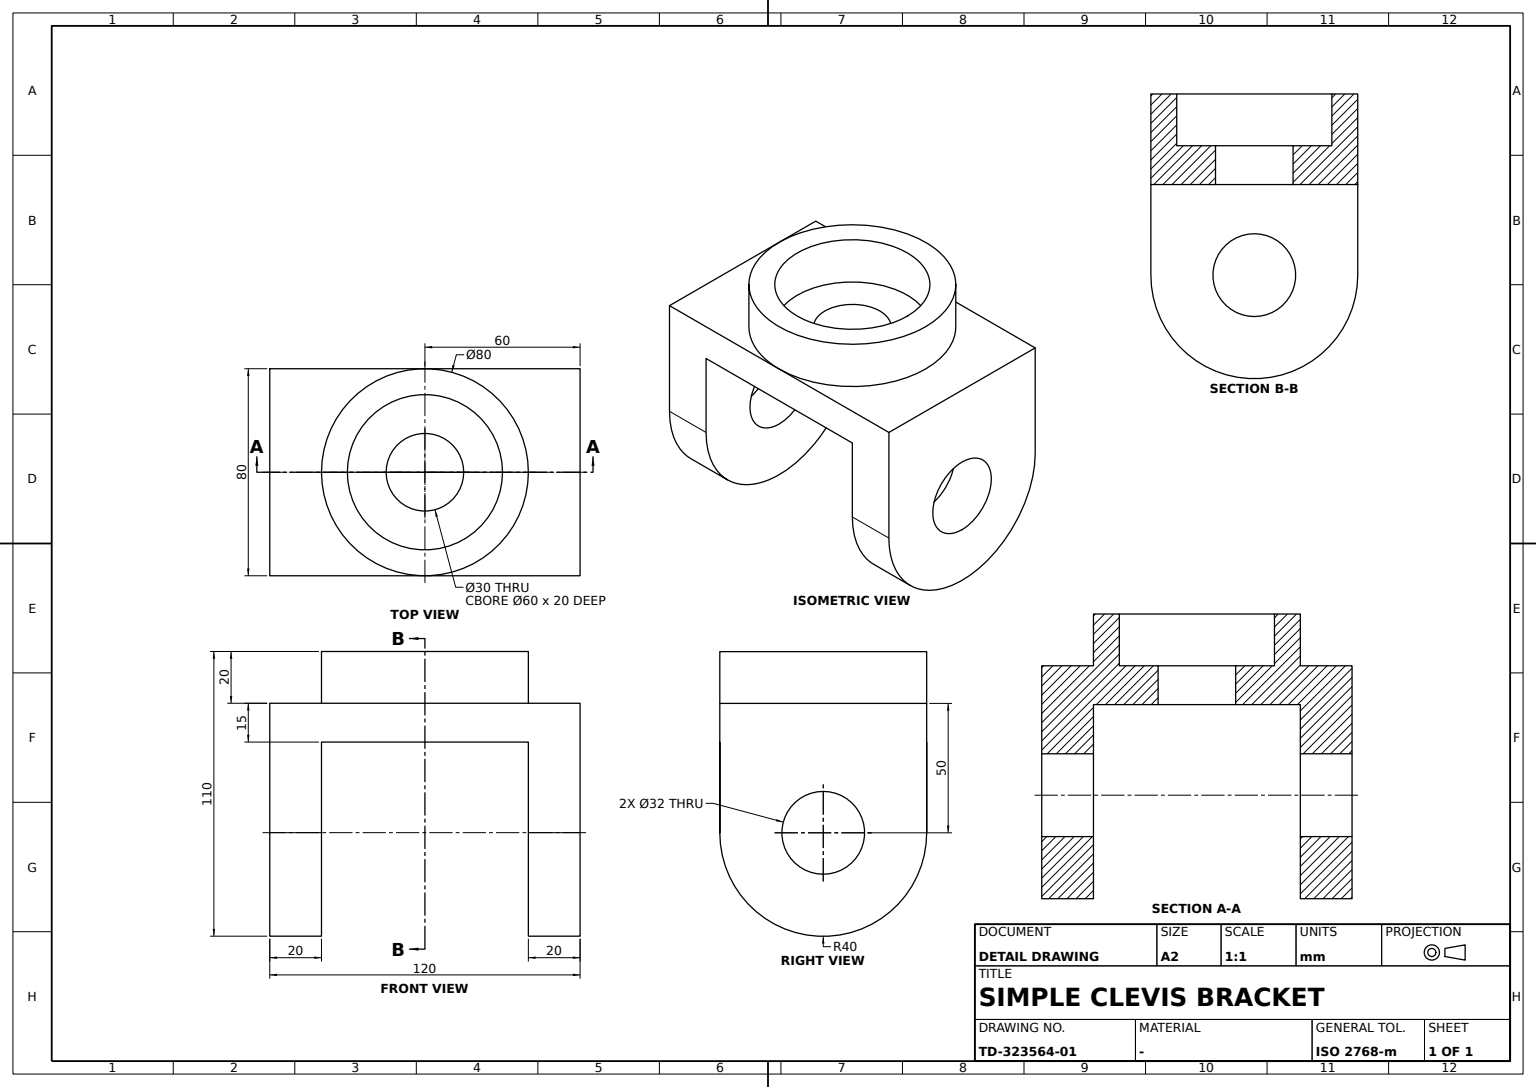
CATIA V5 part; units mm, degrees
sketch "Sketch1" plane through (0, 0, 0) normal (0, 0, 1) x (1, 0, 0)
  line L0 (60, 40) -> (60, -40)
  line L1 (60, -40) -> (-60, -40)
  line L2 (-60, -40) -> (-60, 40)
  line L3 (-60, 40) -> (60, 40)
  dimension "length L0" = 80
  dimension "length L3" = 120
  constraint vertical L0 y-axis
  constraint vertical L2 y-axis
  constraint horizontal L1 x-axis
  constraint horizontal L3 x-axis
  constraint equidistance L0 L2 origin
  constraint equidistance L1 L3 origin
extrude "Pad1" add sketch "Sketch1" along normal blind 15
sketch "Sketch2" plane through (0, 0, 15) normal (0, 0, 1) x (1, 0, 0)
  circle A0 centre (0, 0) radius 40
  circle A1 centre (0, 0) radius 30
  dimension "radius A0" = 40
  dimension "radius A1" = 30
extrude "Pad2" add sketch "Sketch2" along normal blind 20
sketch "Sketch3" plane through (0, 0, 15) normal (0, 0, 1) x (1, 0, 0)
  circle A0 centre (0, 0) radius 15
  dimension "radius A0" = 15
extrude "Pocket1" cut sketch "Sketch3" against normal blind 20
sketch "Sketch4" plane through (60, 0, 0) normal (1, 0, 0) x (0, 1, 0)
  line L0 (-40, 15) -> (40, 15)
  line L1 (40, 15) -> (40, -35)
  line L2 (-40, -35) -> (-40, 15)
  point P0 (-40, -35)
  arc A0 (-40, -35) -> (40, -35) centre (0, -35) ccw
  point P1 (0, -35)
  point P2 (-40, -35)
  circle A1 centre (0, -35) radius 16
  dimension "length L1" = 50
  dimension "radius A1" = 16
  dimension "radius A0" = 40
  dimension "distance y axis P1" = 0
  constraint horizontal L0 x-axis
  constraint vertical L1 y-axis
  constraint vertical L2 y-axis
  constraint tangency A0 L1
  constraint coincidence P0 P2
extrude "Pad3" add sketch "Sketch4" against normal blind 20
mirror "Mirror1" about plane through (0, 0, 0) normal (1, 0, 0) of "Pad3"
